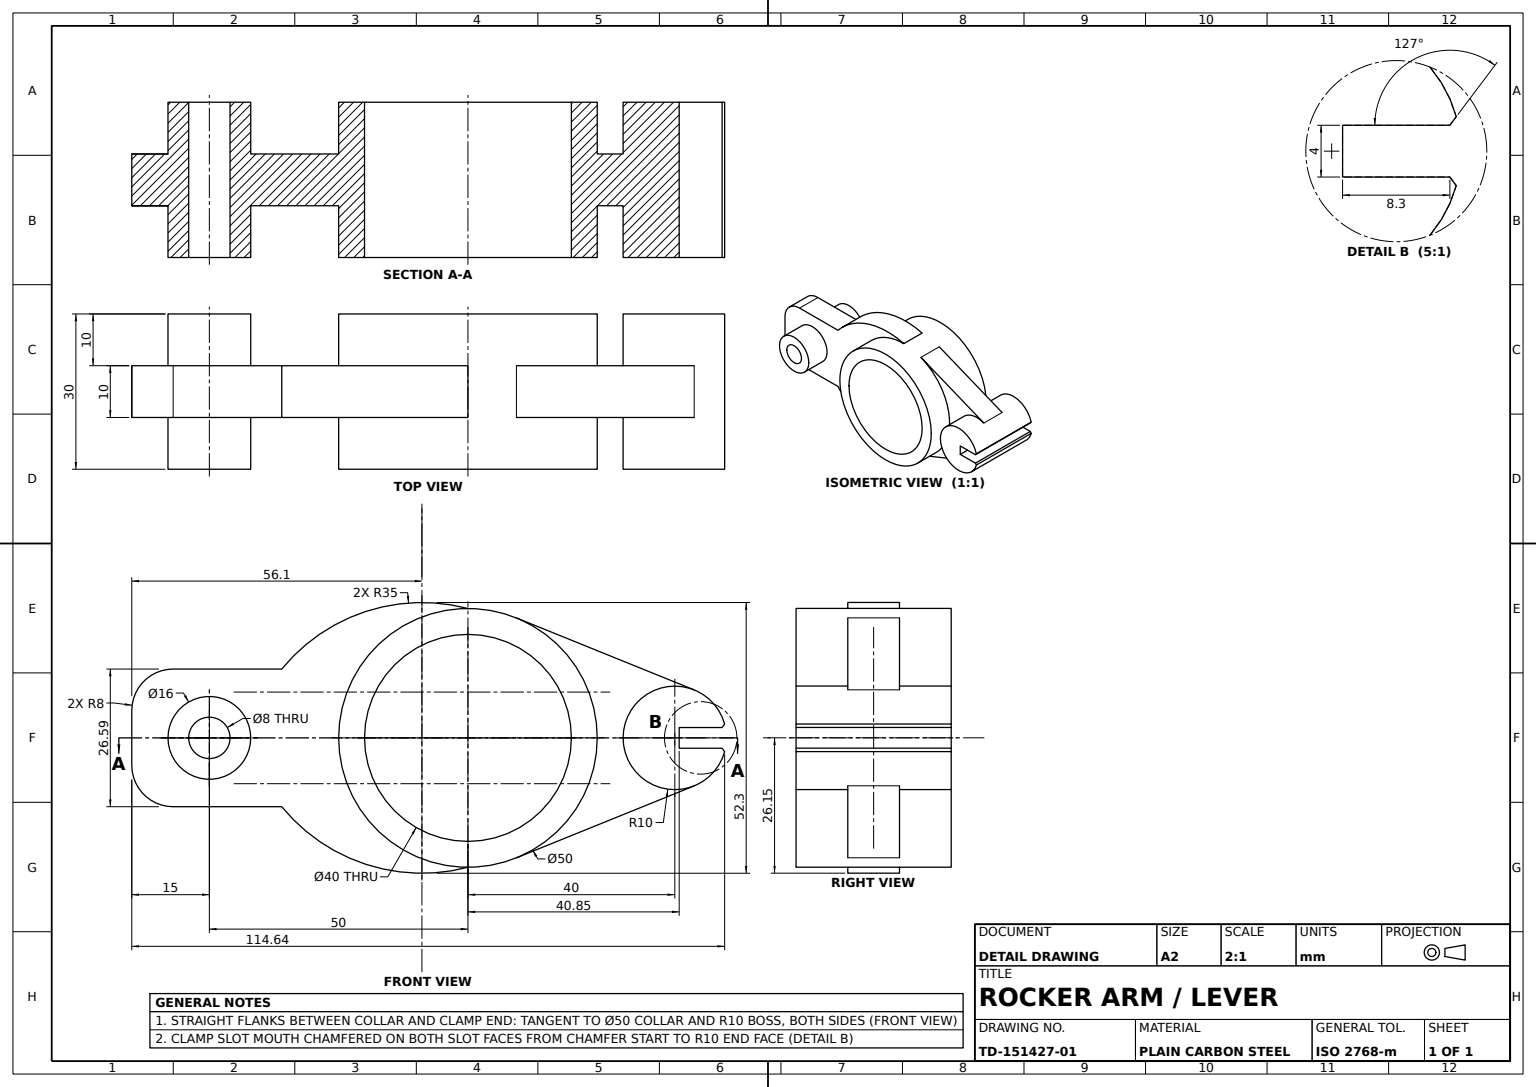
from build123d import *

# Parameters (mm, degrees)
COLLAR_BODY_SKETCH_R   = 25
COLLAR_BODY_DEPTH      = 15
COLLAR_BODY_SKETCH_R_2 = 8
COLLAR_BODY_2_DEPTH    = 15
COLLAR_BODY_SKETCH_R_3 = 10
COLLAR_BODY_3_DEPTH    = 15
LINK_LUGS_DEPTH        = 5
CLAMP_SLOT_SKETCH_R    = 20
CLAMP_SLOT_SKETCH_R_2  = 4
CLAMP_SLOT_CUT_DEPTH   = 77.215631599


with BuildPart() as part:
    # Collar Body Sketch → Collar Body (new, symmetric)
    with BuildSketch(Plane.XY):
        Circle(COLLAR_BODY_SKETCH_R)
    extrude(amount=COLLAR_BODY_DEPTH, both=True)



with BuildPart() as body_2:
    # Collar Body Sketch → Collar Body 2 (new, symmetric)
    with BuildSketch(Plane.XY):
        with Locations((-50, 0)):
            Circle(COLLAR_BODY_SKETCH_R_2)
    extrude(amount=COLLAR_BODY_2_DEPTH, both=True)


with BuildPart() as body_3:
    # Collar Body Sketch → Collar Body 3 (new, symmetric)
    with BuildSketch(Plane.XY):
        with Locations((40, 0)):
            Circle(COLLAR_BODY_SKETCH_R_3)
    extrude(amount=COLLAR_BODY_3_DEPTH, both=True)


with BuildPart() as part_1:
    add(part.part)

    add(body_2.part)  # Link Lugs merges body 2

    add(body_3.part)  # Link Lugs merges body 3
    # Link Lugs Sketch → Link Lugs (add, symmetric)
    with BuildSketch(Plane.XY):
        with BuildLine():
            Line((-65, -5.297031987), (-65, 5.297031987))
            ThreePointArc((-65, 5.297031987), (-62.656854249, 10.953886237), (-57, 13.297031987))
            Line((-57, 13.297031987), (-36, 13.297031987))
            ThreePointArc((-36, 13.297031987), (-19.718668513, 24.43538565), (0, 25))
            ThreePointArc((0, 25), (4.775431561, 24.539666937), (9.375, 23.175620272))
            Line((9.375, 23.175620272), (43.75, 9.270248109))
            ThreePointArc((43.75, 9.270248109), (50, 0), (43.75, -9.270248109))
            Line((43.75, -9.270248109), (9.375, -23.175620272))
            ThreePointArc((9.375, -23.175620272), (4.775431561, -24.539666937), (0, -25))
            ThreePointArc((0, -25), (-19.718668513, -24.43538565), (-36, -13.297031987))
            Line((-36, -13.297031987), (-57, -13.297031987))
            ThreePointArc((-57, -13.297031987), (-62.656854249, -10.953886237), (-65, -5.297031987))
        make_face()
    extrude(amount=LINK_LUGS_DEPTH, both=True)

    # Clamp Slot Sketch → Clamp Slot Cut (cut, through all)
    with BuildSketch(Plane.XY.offset(15)):
        Circle(CLAMP_SLOT_SKETCH_R)
        with Locations((-50, 0)):
            Circle(CLAMP_SLOT_SKETCH_R_2)
        with BuildLine():
            Line((40.845051729, 2), (40.845051729, -2))
            Line((40.845051729, -2), (49.145051729, -2))
            Line((49.145051729, -2), (49.638757615, -2.663522411))
            ThreePointArc((49.638757615, -2.663522411), (50, 0), (49.638757615, 2.663522411))
            Line((49.638757615, 2.663522411), (49.138757615, 2))
            Line((49.138757615, 2), (40.845051729, 2))
        make_face()
    extrude(amount=-CLAMP_SLOT_CUT_DEPTH, mode=Mode.SUBTRACT)


solid = part_1.part
